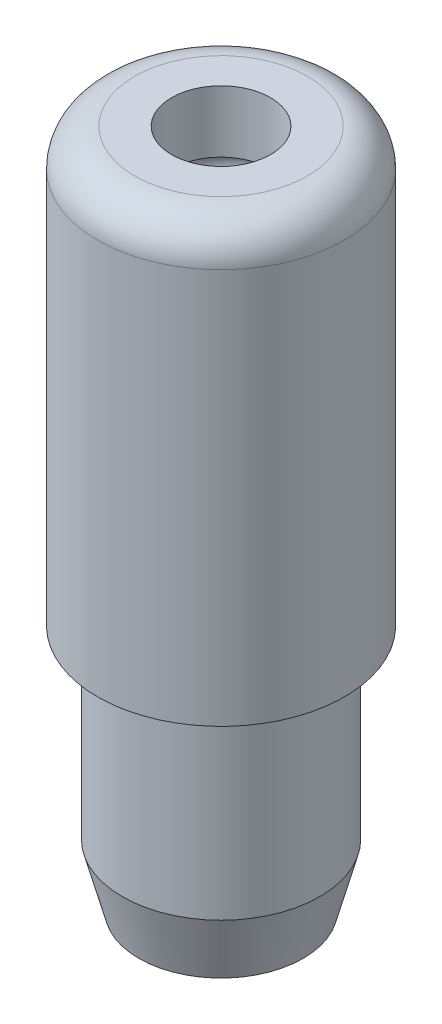
ISO-10303-21;
HEADER;
FILE_DESCRIPTION(('STEP AP214'),'2;1');
FILE_NAME('part.step','',(''),(''),'','','');
FILE_SCHEMA(('AUTOMOTIVE_DESIGN { 1 0 10303 214 1 1 1 1 }'));
ENDSEC;
DATA;
#1=APPLICATION_CONTEXT('core data for automotive mechanical design processes');
#2=APPLICATION_PROTOCOL_DEFINITION('international standard','automotive_design',2000,#1);
#3=PRODUCT_CONTEXT('',#1,'mechanical');
#4=PRODUCT('Part','Part','',(#3));
#5=PRODUCT_RELATED_PRODUCT_CATEGORY('part','',(#4));
#6=PRODUCT_DEFINITION_FORMATION('','',#4);
#7=PRODUCT_DEFINITION_CONTEXT('part definition',#1,'design');
#8=PRODUCT_DEFINITION('design','',#6,#7);
#9=PRODUCT_DEFINITION_SHAPE('','',#8);
#10=(LENGTH_UNIT() NAMED_UNIT(*) SI_UNIT(.MILLI.,.METRE.));
#11=(NAMED_UNIT(*) PLANE_ANGLE_UNIT() SI_UNIT($,.RADIAN.));
#12=(NAMED_UNIT(*) SI_UNIT($,.STERADIAN.) SOLID_ANGLE_UNIT());
#13=UNCERTAINTY_MEASURE_WITH_UNIT(LENGTH_MEASURE(1.E-05),#10,'distance_accuracy_value','');
#14=(GEOMETRIC_REPRESENTATION_CONTEXT(3) GLOBAL_UNCERTAINTY_ASSIGNED_CONTEXT((#13)) GLOBAL_UNIT_ASSIGNED_CONTEXT((#10,
#11,#12)) REPRESENTATION_CONTEXT('',''));
#15=CARTESIAN_POINT('',(0.,0.,0.));
#16=DIRECTION('',(0.,0.,1.));
#17=DIRECTION('',(1.,0.,0.));
#18=AXIS2_PLACEMENT_3D('',#15,#16,#17);
#19=CARTESIAN_POINT('',(6.65000000000001,0.,0.));
#20=DIRECTION('',(0.,1.,0.));
#21=DIRECTION('',(-1.,0.,0.));
#22=AXIS2_PLACEMENT_3D('',#19,#20,#21);
#23=PLANE('',#22);
#24=CARTESIAN_POINT('',(0.,0.,0.));
#25=DIRECTION('',(0.,1.,0.));
#26=DIRECTION('',(-1.,0.,0.));
#27=AXIS2_PLACEMENT_3D('',#24,#25,#26);
#28=CIRCLE('',#27,6.65000000000001);
#29=CARTESIAN_POINT('',(-6.65,0.,0.));
#30=VERTEX_POINT('',#29);
#31=EDGE_CURVE('E10',#30,#30,#28,.T.);
#32=ORIENTED_EDGE('',*,*,#31,.F.);
#33=EDGE_LOOP('',(#32));
#34=FACE_BOUND('',#33,.T.);
#35=CARTESIAN_POINT('',(0.,0.,0.));
#36=DIRECTION('',(0.,1.,0.));
#37=DIRECTION('',(-1.,0.,0.));
#38=AXIS2_PLACEMENT_3D('',#35,#36,#37);
#39=CIRCLE('',#38,5.00000000000001);
#40=CARTESIAN_POINT('',(-5.,0.,0.));
#41=VERTEX_POINT('',#40);
#42=EDGE_CURVE('E81',#41,#41,#39,.T.);
#43=ORIENTED_EDGE('',*,*,#42,.T.);
#44=EDGE_LOOP('',(#43));
#45=FACE_BOUND('',#44,.T.);
#46=ADVANCED_FACE('F40',(#34,#45),#23,.F.);
#47=CARTESIAN_POINT('',(0.,0.,0.));
#48=DIRECTION('',(0.,1.,0.));
#49=DIRECTION('',(-1.,0.,0.));
#50=AXIS2_PLACEMENT_3D('',#47,#48,#49);
#51=CONICAL_SURFACE('',#50,6.65000000000001,0.26179938779915);
#52=CARTESIAN_POINT('',(0.,5.,0.));
#53=DIRECTION('',(0.,1.,0.));
#54=DIRECTION('',(-1.,0.,0.));
#55=AXIS2_PLACEMENT_3D('',#52,#53,#54);
#56=CIRCLE('',#55,7.98974596215562);
#57=CARTESIAN_POINT('',(-7.98974596215562,5.,0.));
#58=VERTEX_POINT('',#57);
#59=EDGE_CURVE('E43',#58,#58,#56,.T.);
#60=ORIENTED_EDGE('',*,*,#59,.F.);
#61=EDGE_LOOP('',(#60));
#62=FACE_BOUND('',#61,.T.);
#63=ORIENTED_EDGE('',*,*,#31,.T.);
#64=EDGE_LOOP('',(#63));
#65=FACE_BOUND('',#64,.T.);
#66=ADVANCED_FACE('F157',(#62,#65),#51,.T.);
#67=CARTESIAN_POINT('',(0.,37.7175572519084,0.));
#68=DIRECTION('',(0.,1.,0.));
#69=DIRECTION('',(-1.,0.,0.));
#70=AXIS2_PLACEMENT_3D('',#67,#68,#69);
#71=CYLINDRICAL_SURFACE('',#70,7.98974596215562);
#72=CARTESIAN_POINT('',(0.,20.,0.));
#73=DIRECTION('',(0.,1.,0.));
#74=DIRECTION('',(-1.,0.,0.));
#75=AXIS2_PLACEMENT_3D('',#72,#73,#74);
#76=CIRCLE('',#75,7.98974596215562);
#77=CARTESIAN_POINT('',(-7.98974596215562,20.,0.));
#78=VERTEX_POINT('',#77);
#79=EDGE_CURVE('E50',#78,#78,#76,.T.);
#80=ORIENTED_EDGE('',*,*,#79,.F.);
#81=EDGE_LOOP('',(#80));
#82=FACE_BOUND('',#81,.T.);
#83=ORIENTED_EDGE('',*,*,#59,.T.);
#84=EDGE_LOOP('',(#83));
#85=FACE_BOUND('',#84,.T.);
#86=ADVANCED_FACE('F153',(#82,#85),#71,.T.);
#87=CARTESIAN_POINT('',(9.98974596215562,20.,0.));
#88=DIRECTION('',(0.,1.,0.));
#89=DIRECTION('',(-1.,0.,0.));
#90=AXIS2_PLACEMENT_3D('',#87,#88,#89);
#91=PLANE('',#90);
#92=CARTESIAN_POINT('',(0.,20.,0.));
#93=DIRECTION('',(0.,1.,0.));
#94=DIRECTION('',(-1.,0.,0.));
#95=AXIS2_PLACEMENT_3D('',#92,#93,#94);
#96=CIRCLE('',#95,9.98974596215562);
#97=CARTESIAN_POINT('',(-9.98974596215562,20.,0.));
#98=VERTEX_POINT('',#97);
#99=EDGE_CURVE('E51',#98,#98,#96,.T.);
#100=ORIENTED_EDGE('',*,*,#99,.F.);
#101=EDGE_LOOP('',(#100));
#102=FACE_BOUND('',#101,.T.);
#103=ORIENTED_EDGE('',*,*,#79,.T.);
#104=EDGE_LOOP('',(#103));
#105=FACE_BOUND('',#104,.T.);
#106=ADVANCED_FACE('F144',(#102,#105),#91,.F.);
#107=CARTESIAN_POINT('',(0.,37.7175572519084,0.));
#108=DIRECTION('',(0.,1.,0.));
#109=DIRECTION('',(-1.,0.,0.));
#110=AXIS2_PLACEMENT_3D('',#107,#108,#109);
#111=CYLINDRICAL_SURFACE('',#110,9.98974596215562);
#112=CARTESIAN_POINT('',(0.,52.,0.));
#113=DIRECTION('',(0.,1.,0.));
#114=DIRECTION('',(-1.,0.,0.));
#115=AXIS2_PLACEMENT_3D('',#112,#113,#114);
#116=CIRCLE('',#115,9.98974596215562);
#117=CARTESIAN_POINT('',(-9.98974596215562,52.,0.));
#118=VERTEX_POINT('',#117);
#119=EDGE_CURVE('E57',#118,#118,#116,.T.);
#120=ORIENTED_EDGE('',*,*,#119,.F.);
#121=EDGE_LOOP('',(#120));
#122=FACE_BOUND('',#121,.T.);
#123=ORIENTED_EDGE('',*,*,#99,.T.);
#124=EDGE_LOOP('',(#123));
#125=FACE_BOUND('',#124,.T.);
#126=ADVANCED_FACE('F137',(#122,#125),#111,.T.);
#127=CARTESIAN_POINT('',(0.,52.,0.));
#128=DIRECTION('',(0.,1.,0.));
#129=DIRECTION('',(-1.,0.,0.));
#130=AXIS2_PLACEMENT_3D('',#127,#128,#129);
#131=TOROIDAL_SURFACE('',#130,6.98974596215562,3.);
#132=CARTESIAN_POINT('',(0.,55.,0.));
#133=DIRECTION('',(0.,1.,0.));
#134=DIRECTION('',(-1.,0.,0.));
#135=AXIS2_PLACEMENT_3D('',#132,#133,#134);
#136=CIRCLE('',#135,6.98974596215562);
#137=CARTESIAN_POINT('',(-6.98974596215562,55.,0.));
#138=VERTEX_POINT('',#137);
#139=EDGE_CURVE('E56',#138,#138,#136,.T.);
#140=ORIENTED_EDGE('',*,*,#139,.F.);
#141=EDGE_LOOP('',(#140));
#142=FACE_BOUND('',#141,.T.);
#143=ORIENTED_EDGE('',*,*,#119,.T.);
#144=EDGE_LOOP('',(#143));
#145=FACE_BOUND('',#144,.T.);
#146=ADVANCED_FACE('F133',(#142,#145),#131,.T.);
#147=CARTESIAN_POINT('',(3.99999999999999,55.,0.));
#148=DIRECTION('',(0.,-1.,0.));
#149=DIRECTION('',(1.,0.,0.));
#150=AXIS2_PLACEMENT_3D('',#147,#148,#149);
#151=PLANE('',#150);
#152=CARTESIAN_POINT('',(0.,55.,0.));
#153=DIRECTION('',(0.,1.,0.));
#154=DIRECTION('',(-1.,0.,0.));
#155=AXIS2_PLACEMENT_3D('',#152,#153,#154);
#156=CIRCLE('',#155,3.99999999999999);
#157=CARTESIAN_POINT('',(-3.99999999999999,55.,0.));
#158=VERTEX_POINT('',#157);
#159=EDGE_CURVE('E65',#158,#158,#156,.T.);
#160=ORIENTED_EDGE('',*,*,#159,.F.);
#161=EDGE_LOOP('',(#160));
#162=FACE_BOUND('',#161,.T.);
#163=ORIENTED_EDGE('',*,*,#139,.T.);
#164=EDGE_LOOP('',(#163));
#165=FACE_BOUND('',#164,.T.);
#166=ADVANCED_FACE('F130',(#162,#165),#151,.F.);
#167=CARTESIAN_POINT('',(0.,37.7175572519084,0.));
#168=DIRECTION('',(0.,1.,0.));
#169=DIRECTION('',(-1.,0.,0.));
#170=AXIS2_PLACEMENT_3D('',#167,#168,#169);
#171=CYLINDRICAL_SURFACE('',#170,3.99999999999999);
#172=CARTESIAN_POINT('',(0.,50.,0.));
#173=DIRECTION('',(0.,1.,0.));
#174=DIRECTION('',(-1.,0.,0.));
#175=AXIS2_PLACEMENT_3D('',#172,#173,#174);
#176=CIRCLE('',#175,3.99999999999999);
#177=CARTESIAN_POINT('',(-3.99999999999999,50.,0.));
#178=VERTEX_POINT('',#177);
#179=EDGE_CURVE('E64',#178,#178,#176,.T.);
#180=ORIENTED_EDGE('',*,*,#179,.F.);
#181=EDGE_LOOP('',(#180));
#182=FACE_BOUND('',#181,.T.);
#183=ORIENTED_EDGE('',*,*,#159,.T.);
#184=EDGE_LOOP('',(#183));
#185=FACE_BOUND('',#184,.T.);
#186=ADVANCED_FACE('F123',(#182,#185),#171,.F.);
#187=CARTESIAN_POINT('',(0.,48.5,0.));
#188=DIRECTION('',(0.,1.,0.));
#189=DIRECTION('',(-1.,0.,0.));
#190=AXIS2_PLACEMENT_3D('',#187,#188,#189);
#191=TOROIDAL_SURFACE('',#190,3.99999999999999,1.5);
#192=CARTESIAN_POINT('',(0.,47.,0.));
#193=DIRECTION('',(0.,1.,0.));
#194=DIRECTION('',(-1.,0.,0.));
#195=AXIS2_PLACEMENT_3D('',#192,#193,#194);
#196=CIRCLE('',#195,3.99999999999999);
#197=CARTESIAN_POINT('',(-3.99999999999999,47.,0.));
#198=VERTEX_POINT('',#197);
#199=EDGE_CURVE('E66',#198,#198,#196,.T.);
#200=ORIENTED_EDGE('',*,*,#199,.F.);
#201=EDGE_LOOP('',(#200));
#202=FACE_BOUND('',#201,.T.);
#203=ORIENTED_EDGE('',*,*,#179,.T.);
#204=EDGE_LOOP('',(#203));
#205=FACE_BOUND('',#204,.T.);
#206=ADVANCED_FACE('F113',(#202,#205),#191,.F.);
#207=CARTESIAN_POINT('',(0.,37.7175572519084,0.));
#208=DIRECTION('',(0.,1.,0.));
#209=DIRECTION('',(-1.,0.,0.));
#210=AXIS2_PLACEMENT_3D('',#207,#208,#209);
#211=CYLINDRICAL_SURFACE('',#210,3.99999999999999);
#212=CARTESIAN_POINT('',(0.,40.,0.));
#213=DIRECTION('',(0.,1.,0.));
#214=DIRECTION('',(-1.,0.,0.));
#215=AXIS2_PLACEMENT_3D('',#212,#213,#214);
#216=CIRCLE('',#215,3.99999999999999);
#217=CARTESIAN_POINT('',(-3.99999999999999,40.,0.));
#218=VERTEX_POINT('',#217);
#219=EDGE_CURVE('E73',#218,#218,#216,.T.);
#220=ORIENTED_EDGE('',*,*,#219,.F.);
#221=EDGE_LOOP('',(#220));
#222=FACE_BOUND('',#221,.T.);
#223=ORIENTED_EDGE('',*,*,#199,.T.);
#224=EDGE_LOOP('',(#223));
#225=FACE_BOUND('',#224,.T.);
#226=ADVANCED_FACE('F107',(#222,#225),#211,.F.);
#227=CARTESIAN_POINT('',(0.,38.5,0.));
#228=DIRECTION('',(0.,1.,0.));
#229=DIRECTION('',(-1.,0.,0.));
#230=AXIS2_PLACEMENT_3D('',#227,#228,#229);
#231=TOROIDAL_SURFACE('',#230,3.99999999999999,1.5);
#232=CARTESIAN_POINT('',(0.,37.,0.));
#233=DIRECTION('',(0.,1.,0.));
#234=DIRECTION('',(-1.,0.,0.));
#235=AXIS2_PLACEMENT_3D('',#232,#233,#234);
#236=CIRCLE('',#235,4.00000000000001);
#237=CARTESIAN_POINT('',(-4.00000000000001,37.,0.));
#238=VERTEX_POINT('',#237);
#239=EDGE_CURVE('E72',#238,#238,#236,.T.);
#240=ORIENTED_EDGE('',*,*,#239,.F.);
#241=EDGE_LOOP('',(#240));
#242=FACE_BOUND('',#241,.T.);
#243=ORIENTED_EDGE('',*,*,#219,.T.);
#244=EDGE_LOOP('',(#243));
#245=FACE_BOUND('',#244,.T.);
#246=ADVANCED_FACE('F104',(#242,#245),#231,.F.);
#247=CARTESIAN_POINT('',(0.,37.7175572519084,0.));
#248=DIRECTION('',(0.,1.,0.));
#249=DIRECTION('',(-1.,0.,0.));
#250=AXIS2_PLACEMENT_3D('',#247,#248,#249);
#251=CYLINDRICAL_SURFACE('',#250,4.00000000000001);
#252=CARTESIAN_POINT('',(0.,28.,0.));
#253=DIRECTION('',(0.,1.,0.));
#254=DIRECTION('',(-1.,0.,0.));
#255=AXIS2_PLACEMENT_3D('',#252,#253,#254);
#256=CIRCLE('',#255,4.00000000000001);
#257=CARTESIAN_POINT('',(-4.00000000000001,28.,0.));
#258=VERTEX_POINT('',#257);
#259=EDGE_CURVE('E77',#258,#258,#256,.T.);
#260=ORIENTED_EDGE('',*,*,#259,.F.);
#261=EDGE_LOOP('',(#260));
#262=FACE_BOUND('',#261,.T.);
#263=ORIENTED_EDGE('',*,*,#239,.T.);
#264=EDGE_LOOP('',(#263));
#265=FACE_BOUND('',#264,.T.);
#266=ADVANCED_FACE('F100',(#262,#265),#251,.F.);
#267=CARTESIAN_POINT('',(0.,28.,0.));
#268=DIRECTION('',(0.,-1.,0.));
#269=DIRECTION('',(1.,0.,0.));
#270=AXIS2_PLACEMENT_3D('',#267,#268,#269);
#271=CONICAL_SURFACE('',#270,4.00000000000001,0.785398163397451);
#272=CARTESIAN_POINT('',(0.,27.,0.));
#273=DIRECTION('',(0.,1.,0.));
#274=DIRECTION('',(-1.,0.,0.));
#275=AXIS2_PLACEMENT_3D('',#272,#273,#274);
#276=CIRCLE('',#275,5.00000000000001);
#277=CARTESIAN_POINT('',(-5.00000000000001,27.,0.));
#278=VERTEX_POINT('',#277);
#279=EDGE_CURVE('E79',#278,#278,#276,.T.);
#280=ORIENTED_EDGE('',*,*,#279,.F.);
#281=EDGE_LOOP('',(#280));
#282=FACE_BOUND('',#281,.T.);
#283=ORIENTED_EDGE('',*,*,#259,.T.);
#284=EDGE_LOOP('',(#283));
#285=FACE_BOUND('',#284,.T.);
#286=ADVANCED_FACE('F91',(#282,#285),#271,.F.);
#287=CARTESIAN_POINT('',(0.,37.7175572519084,0.));
#288=DIRECTION('',(0.,1.,0.));
#289=DIRECTION('',(-1.,0.,0.));
#290=AXIS2_PLACEMENT_3D('',#287,#288,#289);
#291=CYLINDRICAL_SURFACE('',#290,5.00000000000001);
#292=ORIENTED_EDGE('',*,*,#42,.F.);
#293=EDGE_LOOP('',(#292));
#294=FACE_BOUND('',#293,.T.);
#295=ORIENTED_EDGE('',*,*,#279,.T.);
#296=EDGE_LOOP('',(#295));
#297=FACE_BOUND('',#296,.T.);
#298=ADVANCED_FACE('F88',(#294,#297),#291,.F.);
#299=CLOSED_SHELL('',(#46,#66,#86,#106,#126,#146,#166,#186,#206,#226,#246,#266,#286,#298));
#300=MANIFOLD_SOLID_BREP('B2',#299);
#301=ADVANCED_BREP_SHAPE_REPRESENTATION('',(#18,#300),#14);
#302=SHAPE_DEFINITION_REPRESENTATION(#9,#301);
ENDSEC;
END-ISO-10303-21;
